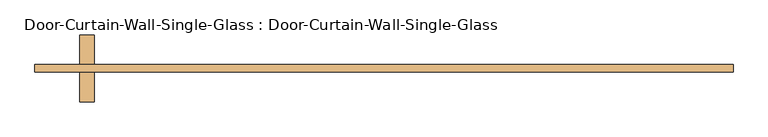
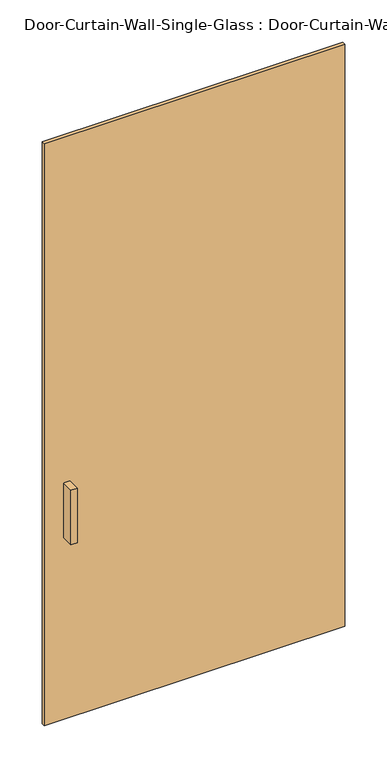
"""IFC4 building model written with IfcOpenShell, lengths in millimetres: door geometry, Door-Curtain-Wall-Single-Glass : Door-Curtain-Wall-Single-Glass."""

from ifc_helpers import new_model, si_unit, frame, origin, origin_with_axes, place, context, project, spatial, polyline, outline, extrude, source, transform, mapped, element, save


def door_curtain_wall_single_glass_door_curtain_wall_single_8a977710(model_context):
    return source(origin(), model_context, "Body", "SweptSolid", [
        extrude(outline(polyline([(595.3125, 50.8), (595.3125, 38.1), (-595.3125, 38.1), (-595.3125, 50.8), (595.3125, 50.8)])), origin_with_axes(), (0.0, 0.0, 1.0), 2438.4),
        extrude(outline(polyline([(-493.7125, -12.7), (-519.1125, -12.7), (-519.1125, 38.1), (-493.7125, 38.1), (-493.7125, -12.7)])), frame((0.0, 0.0, 762.0), z_axis=(0.0, 0.0, 1.0), x_axis=(1.0, 0.0, 0.0)), (0.0, 0.0, 1.0), 228.6),
        extrude(outline(polyline([(-519.1125, 101.6), (-493.7125, 101.6), (-493.7125, 50.8), (-519.1125, 50.8), (-519.1125, 101.6)])), frame((0.0, 0.0, 762.0), z_axis=(0.0, 0.0, 1.0), x_axis=(1.0, 0.0, 0.0)), (0.0, 0.0, 1.0), 228.6),
    ])


if __name__ == "__main__":
    model = new_model("IFC4")
    model_context = context("Model", 3, world=origin())
    ifc_project = project(units=[si_unit("LENGTHUNIT", "METRE", prefix="MILLI")], contexts=[model_context])
    site = spatial("IfcSite", under=ifc_project)
    building = spatial("IfcBuilding", under=site)
    placement = place(None, origin())
    door_curtain_wall_single_glass_door_curtain_wall_single_shape = door_curtain_wall_single_glass_door_curtain_wall_single_8a977710(model_context)
    element("IfcDoor", 1, ObjectType="Door-Curtain-Wall-Single-Glass : Door-Curtain-Wall-Single-Glass", at=placement, inside=building, context=model_context, shape_type="MappedRepresentation", body=[
        mapped(door_curtain_wall_single_glass_door_curtain_wall_single_shape, transform((0.0, 0.0, 0.0), x_axis=(1.0, 0.0, 0.0), y_axis=(0.0, 1.0, 0.0), z_axis=(0.0, 0.0, 1.0))),
    ])
    save(model, "model.ifc")

# Revit data of these elements
# Type "Door-Curtain-Wall-Single-Glass : Door-Curtain-Wall-Single-Glass"
#   Type Mark = "12"
#   Assembly Code = "B2030100"
#   Analytic Construction = "<None>"
#   Width [instance default] = 3' - 0"
#   Thermal Resistance (R) = 10.0000 (h·ft²·°F)/BTU
#   Swing Angle [instance default] = 90.00°
#   Heat Transfer Coefficient (U) = 0.1000 BTU/(h·ft²·°F)
#   Offset = 0' - 2"
#   Define Thermal Properties by = 1
#   Function = 1
#   Door Handle Material = Aluminum
#   Glazing = Glass
#   Visual Light Transmittance = 0
#   Solar Heat Gain Coefficient = 0
#   Construction Type Id = ""
# Element 1 (IfcDoor, "Door-Curtain-Wall-Single-Glass : Door-Curtain-Wall-Single-Glass")
#   Width = 3' - 10 7/8"
#   Materials on its faces: "Aluminum", "Glass"
# Materials
#   "Aluminum": class "Metal", colour RGB 247 247 247, transparency 0, Description = "Aluminum 6061", Cost = 0
#   "Glass": class "Glass", colour RGB 0 128 192, transparency 0.75, Description = "Soda Lime Glass", Cost = 0
